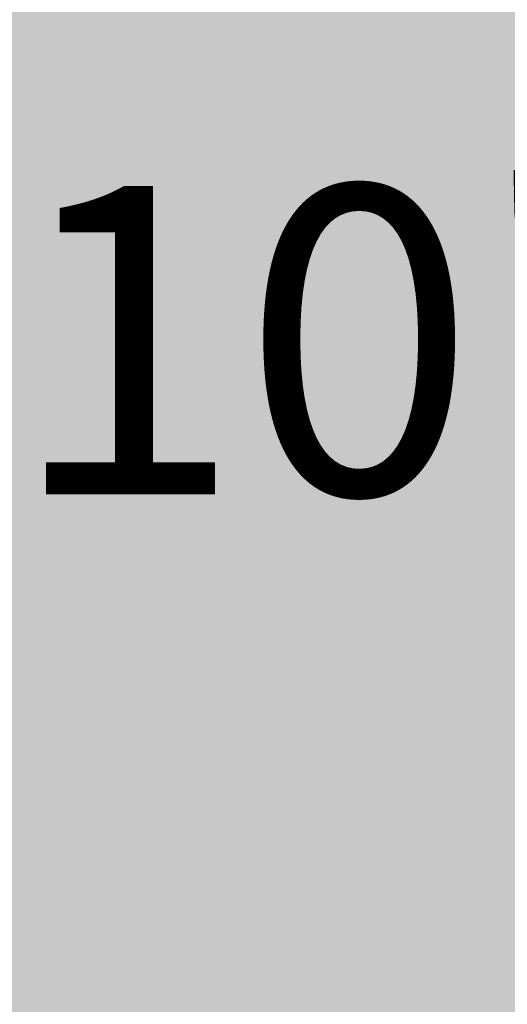
# Model space of a CAD drawing. Units: inches. Extents: x 1704 to 6393, y -157 to 1172.
# Tile 29 of 122: x 2377 to 2398, y 272 to 316. Entities that reach past the tile are written whole.
import ezdxf

# ---------------------------------------------------------------- set-up
doc = ezdxf.new("R2010")
doc.units = ezdxf.units.IN
doc.header["$MEASUREMENT"] = 0
doc.layers.add('A-ANNO-DIMS', color=7, linetype='Continuous', lineweight=13)
doc.layers.add('A-FLOR-PATT', color=7, linetype='Continuous', lineweight=13, true_color=0xf2f2f2)
doc.styles.get("Standard").update_dxf_attribs({"font": 'arial.ttf'})
doc.dimstyles.get("Standard").update_dxf_attribs({"dimtxt": 6, "dimasz": 2, "dimexe": 0.18, "dimexo": 0.0625, "dimgap": 0.09, "dimtad": 0, "dimtih": 1, "dimtoh": 1, "dimdec": 1, "dimzin": 0, "dimdsep": 46, "dimlunit": 3, "dimtxsty": 'Standard', "dimblk": 'ARCHTICK', "dimcen": 0.09, "dimadec": 0, "dimazin": 0, "dimtfac": 1, "dimtdec": 1, "dimtofl": 0, "dimtmove": 0, "dimatfit": 3, "dimfxl": 1, "dimtolj": 1, "dimtzin": 0, "dimarcsym": 0})

# ---------------------------------------------------------------- blocks, each defined once
blk = doc.blocks.new('_ArchTick')
at = {"color": 0, "linetype": 'ByBlock', "const_width": 0.15}
blk.add_lwpolyline([(-0.5, -0.5), (0.5, 0.5)], dxfattribs=at)
blk = doc.blocks.new('*D93')
at = {"layer": 'A-ANNO-DIMS', "color": 0, "lineweight": -2, "transparency": 16777216}
for p, q in [((2605.286, 895.213), (1829.698, 895.213)), ((1829.878, 895.213), (1829.878, 495.866)), ((1829.878, 90.213), (1829.878, 489.56)), ((2605.286, 90.213), (1829.698, 90.213))]:
    blk.add_line(p, q, dxfattribs=at)
at = {"layer": 'Defpoints', "color": 0, "lineweight": -3, "transparency": 16777216}
for p in [(2605.349, 895.213), (1829.878, 90.213), (2605.349, 90.213)]:
    blk.add_point(p, dxfattribs=at)
at = {"layer": 'A-ANNO-DIMS', "color": 0, "lineweight": -2, "transparency": 16777216, "xscale": 2, "yscale": 2, "zscale": 2}
for p, rotation in [((1829.878, 895.213), 90), ((1829.878, 90.213), 270)]:
    blk.add_blockref('_ArchTick', p, dxfattribs=dict(at, rotation=rotation))
at = {"layer": 'A-ANNO-DIMS', "color": 0, "transparency": 16777216, "insert": (1829.878, 492.713), "char_height": 6, "attachment_point": 5}
blk.add_mtext('\\A1;805', dxfattribs=at)

msp = doc.modelspace()

# ---------------------------------------------------------------- hatches: boundary and pattern name
at = {"layer": 'A-FLOR-PATT', "transparency": 33554528}
h = msp.add_hatch(color=256, dxfattribs=at)
h.dxf.hatch_style = 1
h.paths.add_polyline_path([(2325.349, 863.213), (2325.349, 887.213), (2263.349, 887.213), (2167.349, 887.213), (2081.349, 887.213), (2081.349, 719.213), (2277.349, 719.213), (2277.349, 711.213), (2277.349, 372.213), (2349.349, 372.213), (2381.349, 372.213), (2381.349, 364.213), (2353.349, 364.213), (2353.349, 270.213), (2381.349, 270.213), (2381.349, 266.213), (2357.349, 266.213), (2357.349, 98.213), (2381.349, 98.213), (2385.181, 98.213), (2386.482, 98.213), (2424.215, 98.213), (2425.516, 98.213), (2429.349, 98.213), (2597.349, 98.213), (2597.349, 146.213), (2597.349, 218.213), (2597.349, 266.213), (2423.349, 266.213), (2423.349, 270.213), (2473.349, 270.213), (2473.349, 294.213), (2477.349, 294.213), (2477.349, 270.213), (2547.349, 270.213), (2547.349, 364.213), (2477.349, 364.213), (2477.349, 318.213), (2473.349, 318.213), (2473.349, 364.213), (2423.349, 364.213), (2423.349, 372.213), (2469.349, 372.213), (2469.349, 459.213), (2469.349, 538.213), (2350.349, 538.213), (2350.349, 565.713), (2358.349, 565.713), (2358.349, 545.213), (2420.349, 545.213), (2420.349, 610.213), (2358.349, 610.213), (2358.349, 589.713), (2350.349, 589.713), (2350.349, 615.213), (2425.349, 615.213), (2425.349, 607.213), (2425.349, 546.213), (2469.349, 546.213), (2514.349, 546.213), (2514.349, 607.213), (2449.349, 607.213), (2449.349, 615.213), (2451.738, 615.213), (2451.738, 659.213), (2427.738, 659.213), (2427.738, 665.213), (2367.738, 665.213), (2367.738, 667.213), (2367.738, 711.213), (2325.349, 711.213), (2325.349, 719.213), (2325.349, 755.213), (2325.349, 763.213)])
h.paths.add_polyline_path([(2233.858, 822.533, -0.187247), (2233.858, 809.14), (2231.697, 808.804, 0.084893), (2233.131, 814.486), (2230.424, 814.486, -0.104258), (2228.553, 808.313), (2217.751, 807.156, -0.222222), (2217.751, 824.517), (2228.553, 823.359, -0.104258), (2230.424, 817.186), (2233.131, 817.186, 0.084893), (2231.697, 822.868)], flags=16)
h.paths.add_polyline_path([(2213.621, 833.197), (2213.621, 798.475), (2156.048, 798.475), (2156.048, 833.197)], flags=16)
h.paths.add_polyline_path([(2203.932, 848.099), (2205.089, 837.296, -0.222222), (2187.728, 837.296), (2188.885, 848.099, -0.104258), (2195.058, 849.969), (2195.058, 852.676, 0.084893), (2189.377, 851.242), (2189.712, 853.404, -0.187247), (2203.105, 853.404), (2203.44, 851.242, 0.084893), (2197.759, 852.676), (2197.759, 849.969, -0.104258)], flags=16)
h.paths.add_polyline_path([(2181.941, 837.296, -0.222222), (2164.58, 837.296), (2165.737, 848.099, -0.104258), (2171.91, 849.969), (2171.91, 852.676, 0.084893), (2166.229, 851.242), (2166.564, 853.404, -0.187247), (2179.957, 853.404), (2180.292, 851.242, 0.084893), (2174.611, 852.676), (2174.611, 849.969, -0.104258), (2180.784, 848.099)], flags=16)
h.paths.add_polyline_path([(2205.089, 794.376), (2203.932, 783.574, -0.104258), (2197.759, 781.703), (2197.759, 778.996, 0.084893), (2203.44, 780.43), (2203.105, 778.269, -0.187247), (2189.712, 778.269), (2189.377, 780.43, 0.084893), (2195.058, 778.996), (2195.058, 781.703, -0.104258), (2188.885, 783.574), (2187.728, 794.376, -0.222222)], flags=16)
h.paths.add_polyline_path([(2181.941, 794.376), (2180.784, 783.574, -0.104258), (2174.611, 781.703), (2174.611, 778.996, 0.084893), (2180.292, 780.43), (2179.957, 778.269, -0.187247), (2166.564, 778.269), (2166.229, 780.43, 0.084893), (2171.91, 778.996), (2171.91, 781.703, -0.104258), (2165.737, 783.574), (2164.58, 794.376, -0.222222)], flags=16)
h.paths.add_polyline_path([(2151.918, 807.156), (2141.116, 808.313, -0.104258), (2139.245, 814.486), (2136.539, 814.486, 0.084893), (2137.972, 808.804), (2135.811, 809.14, -0.187247), (2135.811, 822.533), (2137.972, 822.868, 0.084893), (2136.539, 817.186), (2139.245, 817.186, -0.104258), (2141.116, 823.359), (2151.918, 824.517, -0.222222)], flags=16)
h.paths.add_polyline_path([(2357.868, 363.41), (2358.814, 363.41, 0.75376)], flags=16)
h.paths.add_polyline_path([(2372.241, 363.117), (2372.248, 363.117), (2372.248, 363.343), (2371.302, 363.343), (2371.302, 363.139, -1.360391)], flags=16)
h.paths.add_polyline_path([(2371.309, 272.716), (2371.302, 272.716), (2371.302, 272.49), (2372.248, 272.49), (2372.248, 272.693, -1.360391)], flags=16)
h.paths.add_polyline_path([(2357.875, 272.716), (2357.868, 272.716), (2357.868, 272.49), (2358.814, 272.49), (2358.814, 272.693, -1.360391)], flags=16)
h.paths.add_polyline_path([(2353.769, 363.074), (2376.347, 363.074), (2376.347, 272.759), (2353.769, 272.759)], flags=16)
h.paths.add_polyline_path([(2354.772, 362.07), (2375.344, 362.07), (2375.344, 273.762), (2354.772, 273.762)], flags=0)
h.paths.add_polyline_path([(2357.868, 363.343), (2358.814, 363.343), (2358.814, 363.117), (2357.868, 363.117)], flags=16)
h.paths.add_polyline_path([(2359.288, 359.184), (2359.288, 360.063), (2370.828, 360.063), (2370.828, 359.184), (2374.332, 359.184), (2374.332, 358.464), (2372.835, 358.464), (2372.835, 357.541), (2374.332, 357.541), (2374.332, 356.82), (2372.835, 356.82), (2372.835, 355.898), (2374.332, 355.898), (2374.332, 355.177), (2372.835, 355.177), (2372.835, 354.254), (2374.332, 354.254), (2374.332, 353.534), (2372.835, 353.534), (2372.835, 352.611), (2374.332, 352.611), (2374.332, 351.89), (2372.835, 351.89), (2372.835, 350.968), (2374.332, 350.968), (2374.332, 350.247), (2372.835, 350.247), (2372.835, 349.324), (2374.332, 349.324), (2374.332, 348.604), (2372.835, 348.604), (2372.835, 347.681), (2374.332, 347.681), (2374.332, 346.96), (2372.835, 346.96), (2372.835, 346.038), (2374.332, 346.038), (2374.332, 345.317), (2372.835, 345.317), (2372.835, 344.395), (2374.332, 344.395), (2374.332, 343.674), (2372.835, 343.674), (2372.835, 342.751), (2374.332, 342.751), (2374.332, 342.03), (2372.835, 342.03), (2372.835, 341.108), (2374.332, 341.108), (2374.332, 340.387), (2372.835, 340.387), (2372.835, 339.465), (2374.332, 339.465), (2374.332, 338.744), (2372.835, 338.744), (2372.835, 337.821), (2374.332, 337.821), (2374.332, 337.1), (2372.835, 337.1), (2372.835, 336.178), (2374.332, 336.178), (2374.332, 335.457), (2372.835, 335.457), (2372.835, 334.535), (2374.332, 334.535), (2374.332, 333.814), (2372.835, 333.814), (2372.835, 332.891), (2374.332, 332.891), (2374.332, 332.171), (2372.835, 332.171), (2372.835, 331.248), (2374.332, 331.248), (2374.332, 330.527), (2372.835, 330.527), (2372.835, 329.605), (2374.332, 329.605), (2374.332, 328.884), (2372.835, 328.884), (2372.835, 327.961), (2374.332, 327.961), (2374.332, 327.241), (2372.835, 327.241), (2372.835, 326.318), (2374.332, 326.318), (2374.332, 325.597), (2372.835, 325.597), (2372.835, 324.675), (2374.332, 324.675), (2374.332, 323.954), (2372.835, 323.954), (2372.835, 323.031), (2374.332, 323.031), (2374.332, 322.311), (2372.835, 322.311), (2372.835, 321.388), (2374.332, 321.388), (2374.332, 320.667), (2372.835, 320.667), (2372.835, 319.745), (2374.332, 319.745), (2374.332, 319.024), (2372.835, 319.024), (2372.835, 318.102), (2374.332, 318.102), (2374.332, 317.381), (2372.835, 317.381), (2372.835, 316.458), (2374.332, 316.458), (2374.332, 315.737), (2372.835, 315.737), (2372.835, 314.815), (2374.332, 314.815), (2374.332, 314.094), (2372.835, 314.094), (2372.835, 313.172), (2374.332, 313.172), (2374.332, 312.451), (2372.835, 312.451), (2372.835, 311.528), (2374.332, 311.528), (2374.332, 310.807), (2372.835, 310.807), (2372.835, 309.885), (2374.332, 309.885), (2374.332, 309.164), (2372.835, 309.164), (2372.835, 308.242), (2374.332, 308.242), (2374.332, 307.521), (2372.835, 307.521), (2372.835, 306.598), (2374.332, 306.598), (2374.332, 305.878), (2372.835, 305.878), (2372.835, 304.955), (2374.332, 304.955), (2374.332, 304.234), (2372.835, 304.234), (2372.835, 303.312), (2374.332, 303.312), (2374.332, 302.591), (2372.835, 302.591), (2372.835, 301.668), (2374.332, 301.668), (2374.332, 300.948), (2372.835, 300.948), (2372.835, 300.025), (2374.332, 300.025), (2374.332, 299.304), (2372.835, 299.304), (2372.835, 298.382), (2374.332, 298.382), (2374.332, 297.661), (2372.835, 297.661), (2372.835, 296.738), (2374.332, 296.738), (2374.332, 296.018), (2372.835, 296.018), (2372.835, 295.095), (2374.332, 295.095), (2374.332, 294.374), (2372.835, 294.374), (2372.835, 293.452), (2374.332, 293.452), (2374.332, 292.731), (2372.835, 292.731), (2372.835, 291.809), (2374.332, 291.809), (2374.332, 291.088), (2372.835, 291.088), (2372.835, 290.165), (2374.332, 290.165), (2374.332, 289.444), (2372.835, 289.444), (2372.835, 288.522), (2374.332, 288.522), (2374.332, 287.801), (2372.835, 287.801), (2372.835, 286.879), (2374.332, 286.879), (2374.332, 286.158), (2372.835, 286.158), (2372.835, 285.235), (2374.332, 285.235), (2374.332, 284.514), (2372.835, 284.514), (2372.835, 283.592), (2374.332, 283.592), (2374.332, 282.871), (2372.835, 282.871), (2372.835, 281.949), (2374.332, 281.949), (2374.332, 281.228), (2372.835, 281.228), (2372.835, 280.305), (2374.332, 280.305), (2374.332, 279.585), (2372.835, 279.585), (2372.835, 278.662), (2374.332, 278.662), (2374.332, 277.941), (2372.835, 277.941), (2372.835, 277.019), (2374.332, 277.019), (2374.332, 276.298), (2370.828, 276.298), (2370.828, 275.769), (2359.288, 275.769), (2359.288, 276.298), (2355.784, 276.298), (2355.784, 277.019), (2357.281, 277.019), (2357.281, 277.941), (2355.784, 277.941), (2355.784, 278.662), (2357.281, 278.662), (2357.281, 279.585), (2355.784, 279.585), (2355.784, 280.305), (2357.281, 280.305), (2357.281, 281.228), (2355.784, 281.228), (2355.784, 281.949), (2357.281, 281.949), (2357.281, 282.871), (2355.784, 282.871), (2355.784, 283.592), (2357.281, 283.592), (2357.281, 284.514), (2355.784, 284.514), (2355.784, 285.235), (2357.281, 285.235), (2357.281, 286.158), (2355.784, 286.158), (2355.784, 286.879), (2357.281, 286.879), (2357.281, 287.801), (2355.784, 287.801), (2355.784, 288.522), (2357.281, 288.522), (2357.281, 289.444), (2355.784, 289.444), (2355.784, 290.165), (2357.281, 290.165), (2357.281, 291.088), (2355.784, 291.088), (2355.784, 291.809), (2357.281, 291.809), (2357.281, 292.731), (2355.784, 292.731), (2355.784, 293.452), (2357.281, 293.452), (2357.281, 294.374), (2355.784, 294.374), (2355.784, 295.095), (2357.281, 295.095), (2357.281, 296.018), (2355.784, 296.018), (2355.784, 296.738), (2357.281, 296.738), (2357.281, 297.661), (2355.784, 297.661), (2355.784, 298.382), (2357.281, 298.382), (2357.281, 299.304), (2355.784, 299.304), (2355.784, 300.025), (2357.281, 300.025), (2357.281, 300.948), (2355.784, 300.948), (2355.784, 301.668), (2357.281, 301.668), (2357.281, 302.591), (2355.784, 302.591), (2355.784, 303.312), (2357.281, 303.312), (2357.281, 304.234), (2355.784, 304.234), (2355.784, 304.955), (2357.281, 304.955), (2357.281, 305.878), (2355.784, 305.878), (2355.784, 306.598), (2357.281, 306.598), (2357.281, 307.521), (2355.784, 307.521), (2355.784, 308.242), (2357.281, 308.242), (2357.281, 309.164), (2355.784, 309.164), (2355.784, 309.885), (2357.281, 309.885), (2357.281, 310.807), (2355.784, 310.807), (2355.784, 311.528), (2357.281, 311.528), (2357.281, 312.451), (2355.784, 312.451), (2355.784, 313.172), (2357.281, 313.172), (2357.281, 314.094), (2355.784, 314.094), (2355.784, 314.815), (2357.281, 314.815), (2357.281, 315.737), (2355.784, 315.737), (2355.784, 316.458), (2357.281, 316.458), (2357.281, 317.381), (2355.784, 317.381), (2355.784, 318.102), (2357.281, 318.102), (2357.281, 319.024), (2355.784, 319.024), (2355.784, 319.745), (2357.281, 319.745), (2357.281, 320.667), (2355.784, 320.667), (2355.784, 321.388), (2357.281, 321.388), (2357.281, 322.311), (2355.784, 322.311), (2355.784, 323.031), (2357.281, 323.031), (2357.281, 323.954), (2355.784, 323.954), (2355.784, 324.675), (2357.281, 324.675), (2357.281, 325.597), (2355.784, 325.597), (2355.784, 326.318), (2357.281, 326.318), (2357.281, 327.241), (2355.784, 327.241), (2355.784, 327.961), (2357.281, 327.961), (2357.281, 328.884), (2355.784, 328.884), (2355.784, 329.605), (2357.281, 329.605), (2357.281, 330.527), (2355.784, 330.527), (2355.784, 331.248), (2357.281, 331.248), (2357.281, 332.171), (2355.784, 332.171), (2355.784, 332.891), (2357.281, 332.891), (2357.281, 333.814), (2355.784, 333.814), (2355.784, 334.535), (2357.281, 334.535), (2357.281, 335.457), (2355.784, 335.457), (2355.784, 336.178), (2357.281, 336.178), (2357.281, 337.1), (2355.784, 337.1), (2355.784, 337.821), (2357.281, 337.821), (2357.281, 338.744), (2355.784, 338.744), (2355.784, 339.465), (2357.281, 339.465), (2357.281, 340.387), (2355.784, 340.387), (2355.784, 341.108), (2357.281, 341.108), (2357.281, 342.03), (2355.784, 342.03), (2355.784, 342.751), (2357.281, 342.751), (2357.281, 343.674), (2355.784, 343.674), (2355.784, 344.395), (2357.281, 344.395), (2357.281, 345.317), (2355.784, 345.317), (2355.784, 346.038), (2357.281, 346.038), (2357.281, 346.96), (2355.784, 346.96), (2355.784, 347.681), (2357.281, 347.681), (2357.281, 348.604), (2355.784, 348.604), (2355.784, 349.324), (2357.281, 349.324), (2357.281, 350.247), (2355.784, 350.247), (2355.784, 350.968), (2357.281, 350.968), (2357.281, 351.89), (2355.784, 351.89), (2355.784, 352.611), (2357.281, 352.611), (2357.281, 353.534), (2355.784, 353.534), (2355.784, 354.254), (2357.281, 354.254), (2357.281, 355.177), (2355.784, 355.177), (2355.784, 355.898), (2357.281, 355.898), (2357.281, 356.82), (2355.784, 356.82), (2355.784, 357.541), (2357.281, 357.541), (2357.281, 358.464), (2355.784, 358.464), (2355.784, 359.184)], flags=0)

# ---------------------------------------------------------------- texts
at = {"layer": 'A-ANNO-DIMS'}
msp.add_text('10\' 0" X 7\' 10"', height=13.6672, dxfattribs=at).set_placement((2376.347, 295.054))

# ---------------------------------------------------------------- dimensions: what is measured, and where the dimension line sits
dim = msp.add_linear_dim(base=(1829.878, 90.213), p1=(2605.349, 895.213), p2=(2605.349, 90.213), angle=90, dimstyle='Standard', override={"dimdec": 0, "dimlfac": 1, "dimrnd": 0, "dimzin": 0, "dimdsep": 46, "dimlunit": 2}, dxfattribs=at)
dim.commit()
dim.dimension.update_dxf_attribs({"geometry": '*D93', "text_midpoint": (1829.878, 492.713)})

doc.saveas('drawing.dxf')
